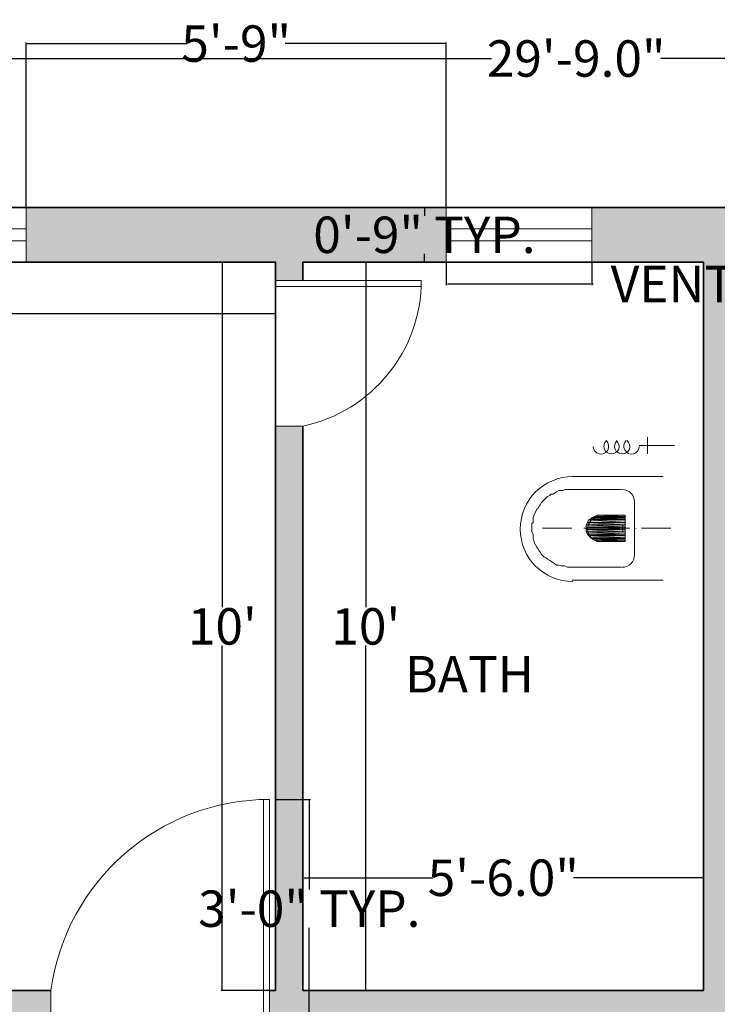
# Model space of a CAD drawing. Units: inches. Extents: x 302 to 1258, y 831 to 1373.
# Tile 4 of 13: x 455 to 569, y 1211 to 1373. Entities that reach past the tile are written whole.
import ezdxf

# ---------------------------------------------------------------- set-up
doc = ezdxf.new("R2010")
doc.units = ezdxf.units.IN
doc.header["$MEASUREMENT"] = 0
for name, color, linetype, lineweight in [('A-ANNO-DIMS', 2, 'Continuous', 18), ('A-AREA-IDEN', 7, 'Continuous', 18), ('A-DOOR', 3, 'Continuous', 18), ('A-FLOR-FIXT', 8, 'Continuous', 18), ('A-GLAZ', 4, 'Continuous', 18), ('A-WALL', 7, 'Continuous', 35), ('A-WALL-PATT', 251, 'Continuous', 13)]:
    doc.layers.add(name, color=color, linetype=linetype, lineweight=lineweight)
doc.styles.get("Standard").update_dxf_attribs({"font": 'arial.ttf'})
doc.dimstyles.get("Standard").update_dxf_attribs({"dimtxt": 6, "dimasz": 0.18, "dimexe": 0.18, "dimexo": 0.0625, "dimgap": 0.09, "dimtad": 0, "dimtih": 1, "dimtoh": 1, "dimdec": 1, "dimzin": 0, "dimdsep": 46, "dimlunit": 3, "dimtxsty": 'Standard', "dimcen": 0.09, "dimadec": 0, "dimazin": 0, "dimtfac": 1, "dimtdec": 1, "dimtofl": 0, "dimtmove": 0, "dimatfit": 3, "dimfxl": 1, "dimtolj": 1, "dimtzin": 0, "dimarcsym": 0})

# ---------------------------------------------------------------- blocks, each defined once
blk = doc.blocks.new('*D3')
at = {"layer": 'A-ANNO-DIMS', "color": 0, "lineweight": -2, "transparency": 16777216}
for p, q in [((376.67, 1333.26), (376.67, 1324.65)), ((496.67, 1333.26), (496.67, 1324.65)), ((376.85, 1324.83), (431.77, 1324.83)), ((496.49, 1324.83), (441.57, 1324.83))]:
    blk.add_line(p, q, dxfattribs=at)
at = {"layer": 'A-ANNO-DIMS', "color": 0, "transparency": 16777216}
for points in [[(376.85, 1324.86), (376.85, 1324.8), (376.67, 1324.83)], [(496.49, 1324.86), (496.49, 1324.8), (496.67, 1324.83)]]:
    blk.add_solid(points, dxfattribs=at)
at = {"layer": 'Defpoints', "color": 0, "transparency": 16777216}
for p in [(376.67, 1333.32), (496.67, 1333.32), (496.67, 1324.83)]:
    blk.add_point(p, dxfattribs=at)
at = {"layer": 'A-ANNO-DIMS', "color": 0, "transparency": 16777216, "insert": (436.67, 1324.83), "char_height": 6, "attachment_point": 5}
blk.add_mtext("\\A1;10'", dxfattribs=at)
blk = doc.blocks.new('*D4')
at = {"layer": 'A-ANNO-DIMS', "color": 0, "lineweight": -2, "transparency": 16777216}
for p, q in [((501.17, 1213.38), (501.17, 1232.1)), ((501.35, 1231.92), (522.61, 1231.92)), ((566.99, 1231.92), (545.73, 1231.92)), ((567.17, 1213.38), (567.17, 1232.1))]:
    blk.add_line(p, q, dxfattribs=at)
at = {"layer": 'A-ANNO-DIMS', "color": 0, "transparency": 16777216}
for points in [[(501.35, 1231.95), (501.35, 1231.89), (501.17, 1231.92)], [(566.99, 1231.95), (566.99, 1231.89), (567.17, 1231.92)]]:
    blk.add_solid(points, dxfattribs=at)
at = {"layer": 'Defpoints', "color": 0, "transparency": 16777216}
for p in [(567.17, 1231.92), (501.17, 1213.32), (567.17, 1213.32)]:
    blk.add_point(p, dxfattribs=at)
at = {"layer": 'A-ANNO-DIMS', "color": 0, "transparency": 16777216, "insert": (534.17, 1231.92), "char_height": 6, "attachment_point": 5}
blk.add_mtext('\\A1;5\'-6.0"', dxfattribs=at)
blk = doc.blocks.new('*D5')
at = {"layer": 'A-ANNO-DIMS', "color": 0, "lineweight": -2, "transparency": 16777216}
for p, q in [((496.61, 1333.32), (487.71, 1333.32)), ((487.89, 1333.14), (487.89, 1276.47)), ((487.89, 1213.5), (487.89, 1270.17)), ((496.61, 1213.32), (487.71, 1213.32))]:
    blk.add_line(p, q, dxfattribs=at)
at = {"layer": 'A-ANNO-DIMS', "color": 0, "transparency": 16777216}
for points in [[(487.86, 1333.14), (487.92, 1333.14), (487.89, 1333.32)], [(487.86, 1213.5), (487.92, 1213.5), (487.89, 1213.32)]]:
    blk.add_solid(points, dxfattribs=at)
at = {"layer": 'Defpoints', "color": 0, "transparency": 16777216}
for p in [(496.67, 1333.32), (487.89, 1213.32), (496.67, 1213.32)]:
    blk.add_point(p, dxfattribs=at)
at = {"layer": 'A-ANNO-DIMS', "color": 0, "transparency": 16777216, "insert": (487.89, 1273.32), "char_height": 6, "attachment_point": 5}
blk.add_mtext("\\A1;10'", dxfattribs=at)
blk = doc.blocks.new('*D6')
at = {"layer": 'A-ANNO-DIMS', "color": 0, "lineweight": -2, "transparency": 16777216}
for p, q in [((567.11, 1333.32), (511.34, 1333.32)), ((511.52, 1333.14), (511.52, 1276.47)), ((511.52, 1213.5), (511.52, 1270.17)), ((567.11, 1213.32), (511.34, 1213.32))]:
    blk.add_line(p, q, dxfattribs=at)
at = {"layer": 'A-ANNO-DIMS', "color": 0, "transparency": 16777216}
for points in [[(511.49, 1333.14), (511.55, 1333.14), (511.52, 1333.32)], [(511.49, 1213.5), (511.55, 1213.5), (511.52, 1213.32)]]:
    blk.add_solid(points, dxfattribs=at)
at = {"layer": 'Defpoints', "color": 0, "transparency": 16777216}
for p in [(567.17, 1333.32), (511.52, 1213.32), (567.17, 1213.32)]:
    blk.add_point(p, dxfattribs=at)
at = {"layer": 'A-ANNO-DIMS', "color": 0, "transparency": 16777216, "insert": (511.52, 1273.32), "char_height": 6, "attachment_point": 5}
blk.add_mtext("\\A1;10'", dxfattribs=at)
blk = doc.blocks.new('*D31')
at = {"layer": 'A-ANNO-DIMS', "color": 0, "lineweight": -2, "transparency": 16777216}
for p, q in [((367.67, 1342.38), (367.67, 1367.04)), ((367.85, 1366.86), (532.23, 1366.86)), ((724.49, 1366.86), (560.11, 1366.86)), ((724.67, 1342.38), (724.67, 1367.04))]:
    blk.add_line(p, q, dxfattribs=at)
at = {"layer": 'A-ANNO-DIMS', "color": 0, "transparency": 16777216}
for points in [[(367.85, 1366.89), (367.85, 1366.83), (367.67, 1366.86)], [(724.49, 1366.89), (724.49, 1366.83), (724.67, 1366.86)]]:
    blk.add_solid(points, dxfattribs=at)
at = {"layer": 'Defpoints', "color": 0, "transparency": 16777216}
for p in [(724.67, 1366.86), (367.67, 1342.32), (724.67, 1342.32)]:
    blk.add_point(p, dxfattribs=at)
at = {"layer": 'A-ANNO-DIMS', "color": 0, "transparency": 16777216, "insert": (546.17, 1366.86), "char_height": 6, "attachment_point": 5}
blk.add_mtext('\\A1;29\'-9.0"', dxfattribs=at)
blk = doc.blocks.new('WC-PLAN')
h = blk.add_hatch(color=256)
h.paths.add_polyline_path([(17.3, 10.16), (11.23, 10.16), (17.3, 9.71)])
h.paths.add_polyline_path([(11.23, 10.16), (17.3, 9.71), (11.08, 9.71)])
h = blk.add_hatch(color=256)
h.paths.add_polyline_path([(17.3, 10.32), (11.61, 10.32), (17.3, 10.16)])
h.paths.add_polyline_path([(11.61, 10.32), (17.3, 10.16), (11.23, 10.16)])
h = blk.add_hatch(color=256)
h.paths.add_polyline_path([(17.3, 10.54), (11.83, 10.54), (17.3, 10.32)])
h.paths.add_polyline_path([(11.83, 10.54), (17.3, 10.32), (11.61, 10.32)])
h = blk.add_hatch(color=256)
h.paths.add_polyline_path([(17.3, 10.7), (12.21, 10.7), (17.3, 10.54)])
h.paths.add_polyline_path([(12.21, 10.7), (17.3, 10.54), (11.83, 10.54)])
h = blk.add_hatch(color=256)
h.paths.add_polyline_path([(17.3, 10.92), (12.59, 10.92), (17.3, 10.7)])
h.paths.add_polyline_path([(12.59, 10.92), (17.3, 10.7), (12.21, 10.7)])
h = blk.add_hatch(color=256)
h.paths.add_polyline_path([(17.3, 9.71), (11.08, 9.71), (17.3, 9.33)])
h.paths.add_polyline_path([(11.08, 9.71), (17.3, 9.33), (10.85, 9.33)])
h = blk.add_hatch(color=256)
h.paths.add_polyline_path([(17.3, 9.33), (10.85, 9.33), (17.3, 8.95)])
h.paths.add_polyline_path([(10.85, 9.33), (17.3, 8.95), (10.85, 8.95)])
h = blk.add_hatch(color=256)
h.paths.add_polyline_path([(17.3, 8.95), (10.85, 8.95), (17.3, 8.57)])
h.paths.add_polyline_path([(10.85, 8.95), (17.3, 8.57), (10.85, 8.57)])
h = blk.add_hatch(color=256)
h.paths.add_polyline_path([(17.3, 8.57), (10.85, 8.57), (17.3, 8.19)])
h.paths.add_polyline_path([(10.85, 8.57), (17.3, 8.19), (10.85, 8.19)])
h = blk.add_hatch(color=256)
h.paths.add_polyline_path([(17.3, 8.19), (10.85, 8.19), (17.3, 7.81)])
h.paths.add_polyline_path([(10.85, 8.19), (17.3, 7.81), (11.08, 7.81)])
h = blk.add_hatch(color=256)
h.paths.add_polyline_path([(17.3, 7.81), (11.08, 7.81), (17.3, 7.59)])
h.paths.add_polyline_path([(11.08, 7.81), (17.3, 7.59), (11.23, 7.59)])
h = blk.add_hatch(color=256)
h.paths.add_polyline_path([(17.3, 7.59), (11.23, 7.59), (17.3, 7.21)])
h.paths.add_polyline_path([(11.23, 7.59), (17.3, 7.21), (11.61, 7.21)])
h = blk.add_hatch(color=256)
h.paths.add_polyline_path([(17.3, 7.21), (11.61, 7.21), (17.3, 7.05)])
h.paths.add_polyline_path([(11.61, 7.21), (17.3, 7.05), (11.83, 7.05)])
h = blk.add_hatch(color=256)
h.paths.add_polyline_path([(17.3, 7.05), (11.83, 7.05), (17.3, 6.83)])
h.paths.add_polyline_path([(11.83, 7.05), (17.3, 6.83), (12.21, 6.83)])
h = blk.add_hatch(color=256)
h.paths.add_polyline_path([(17.3, 6.83), (12.21, 6.83), (17.3, 6.6)])
h.paths.add_polyline_path([(12.21, 6.83), (17.3, 6.6), (12.59, 6.6)])
h.paths.add_polyline_path([(17.3, 6.6), (12.59, 6.6), (12.97, 6.6)])
for points in [[(20.94, 21.03), (20.94, 23.77), (20.94, 23.77)], [(25.41, 22.4), (19.57, 22.4), (19.57, 22.4)], [(23.52, 17.3), (8.5, 17.3), (8.5, 17.3)], [(9.48, 2.35), (8.72, 2.35), (8.12, 2.35), (7.74, 2.35), (7.36, 2.58), (6.98, 2.58), (6.75, 2.58), (6.37, 2.73), (5.99, 2.73), (5.61, 2.96), (5.39, 3.11), (5.01, 3.34), (4.85, 3.49), (4.48, 3.72), (4.25, 3.94), (3.87, 4.1), (3.64, 4.32), (3.49, 4.48), (3.26, 4.85), (3.11, 5.08), (2.88, 5.46), (2.73, 5.69), (2.5, 6.07), (2.28, 6.45), (2.28, 6.6), (2.12, 7.05), (2.12, 7.43), (2.12, 7.81), (1.9, 8.19), (1.9, 8.8), (1.9, 9.56), (2.12, 9.71), (2.12, 10.16), (2.12, 10.54), (2.28, 10.92), (2.28, 11.07), (2.5, 11.45), (2.73, 11.91), (2.88, 12.06), (3.11, 12.44), (3.26, 12.67), (3.49, 13.05), (3.64, 13.2), (3.87, 13.43), (4.25, 13.81), (4.48, 14.03), (4.85, 14.18), (5.01, 14.41), (5.39, 14.41), (5.61, 14.56), (5.99, 14.79), (6.37, 15.02), (6.75, 15.02), (6.98, 15.02), (7.36, 15.17), (7.74, 15.17), (8.12, 15.17), (8.72, 15.17), (9.48, 15.17)], [(16.69, 15.17), (9.48, 15.17), (9.48, 15.17)], [(18.81, 4.48), (18.81, 13.2), (18.81, 13.2)], [(17.3, 10.92), (12.97, 10.92), (12.97, 10.92)], [(17.3, 6.6), (17.3, 10.92), (17.3, 10.92)], [(8.5, 8.8), (3.64, 8.8), (3.64, 8.8)], [(18.05, 8.8), (10.47, 8.8), (10.47, 8.8)], [(16.84, 9.18), (16.92, 9.18), (16.92, 9.18)], [(16.84, 8.8), (16.84, 8.95), (16.84, 9.18)], [(16.84, 8.8), (16.92, 8.72), (16.92, 8.72)], [(16.84, 8.34), (16.84, 8.57), (16.84, 8.8)], [(16.84, 8.34), (16.92, 8.34), (16.92, 8.34)], [(19.04, 8.8), (19.04, 8.72), (19.04, 8.72)], [(24.81, 8.8), (19.95, 8.8), (19.95, 8.8)], [(17.3, 6.6), (12.97, 6.6), (12.97, 6.6)], [(16.69, 2.35), (9.48, 2.35), (9.48, 2.35)], [(23.52, 0.23), (8.5, 0.23), (8.5, 0.23)]]:
    blk.add_lwpolyline(points)
for points in [[(11.23, 10.16), (17.3, 9.71), (11.08, 9.71)], [(11.61, 10.32), (17.3, 10.16), (11.23, 10.16)], [(17.3, 10.16), (11.23, 10.16), (17.3, 9.71)], [(11.83, 10.54), (17.3, 10.32), (11.61, 10.32)], [(17.3, 10.32), (11.61, 10.32), (17.3, 10.16)], [(12.21, 10.7), (17.3, 10.54), (11.83, 10.54)], [(17.3, 10.54), (11.83, 10.54), (17.3, 10.32)], [(12.59, 10.92), (17.3, 10.7), (12.21, 10.7)], [(17.3, 10.7), (12.21, 10.7), (17.3, 10.54)], [(12.97, 10.92), (17.3, 10.92), (12.59, 10.92)], [(17.3, 10.92), (12.59, 10.92), (17.3, 10.7)], [(17.3, 10.92), (12.97, 10.92)], [(11.08, 9.71), (17.3, 9.33), (10.85, 9.33)], [(17.3, 9.33), (10.85, 9.33), (17.3, 8.95)], [(10.85, 9.33), (17.3, 8.95), (10.85, 8.95)], [(17.3, 8.95), (10.85, 8.95), (17.3, 8.57)], [(10.85, 8.95), (17.3, 8.57), (10.85, 8.57)], [(17.3, 8.57), (10.85, 8.57), (17.3, 8.19)], [(10.85, 8.57), (17.3, 8.19), (10.85, 8.19)], [(17.3, 8.19), (10.85, 8.19), (17.3, 7.81)], [(10.85, 8.19), (17.3, 7.81), (11.08, 7.81)], [(17.3, 9.71), (11.08, 9.71), (17.3, 9.33)], [(17.3, 7.81), (11.08, 7.81), (17.3, 7.59)], [(11.08, 7.81), (17.3, 7.59), (11.23, 7.59)], [(17.3, 7.59), (11.23, 7.59), (17.3, 7.21)], [(11.23, 7.59), (17.3, 7.21), (11.61, 7.21)], [(17.3, 7.21), (11.61, 7.21), (17.3, 7.05)], [(11.61, 7.21), (17.3, 7.05), (11.83, 7.05)], [(17.3, 7.05), (11.83, 7.05), (17.3, 6.83)], [(11.83, 7.05), (17.3, 6.83), (12.21, 6.83)], [(17.3, 6.83), (12.21, 6.83), (17.3, 6.6)], [(12.21, 6.83), (17.3, 6.6), (12.59, 6.6)], [(17.3, 6.6), (12.59, 6.6), (12.97, 6.6)], [(12.59, 6.6), (17.3, 6.6), (17.3, 6.6)]]:
    blk.add_lwpolyline(points, close=True)
for points, knots in [([(11.99, 22.25), (11.99, 21.72), (12.44, 21.19), (12.97, 21.03), (12.97, 21.03), (13.5, 20.88), (14.11, 21.19), (14.41, 21.64), (14.41, 21.64), (14.64, 22.17), (14.56, 22.78), (14.19, 23.16)], [0, 0, 0, 0, 0.083333, 0.083333, 0.083333, 0.083334, 0.166667, 0.166667, 0.166667, 0.166668, 1, 1, 1, 1]), ([(14.19, 23.23), (13.81, 22.86), (13.65, 22.32), (13.88, 21.79), (13.88, 21.79), (14.03, 21.34), (14.49, 21.03), (15.02, 21.03), (15.02, 21.03), (15.55, 21.03), (16.01, 21.34), (16.23, 21.79), (16.23, 21.79), (16.39, 22.32), (16.23, 22.86), (15.85, 23.23)], [0, 0, 0, 0, 0.0625, 0.0625, 0.0625, 0.062501, 0.125, 0.125, 0.125, 0.125001, 0.1875, 0.1875, 0.1875, 0.187501, 1, 1, 1, 1]), ([(15.93, 23.16), (15.55, 22.86), (15.4, 22.25), (15.63, 21.79), (15.63, 21.79), (15.78, 21.34), (16.31, 21.03), (16.76, 21.03), (16.76, 21.03), (17.3, 21.03), (17.75, 21.34), (17.98, 21.79), (17.98, 21.79), (18.13, 22.32), (17.98, 22.86), (17.6, 23.23)], [0, 0, 0, 0, 0.0625, 0.0625, 0.0625, 0.062501, 0.125, 0.125, 0.125, 0.125001, 0.1875, 0.1875, 0.1875, 0.187501, 1, 1, 1, 1]), ([(17.45, 23.23), (17.07, 22.86), (16.92, 22.17), (17.22, 21.72), (17.22, 21.72), (17.52, 21.19), (18.05, 20.88), (18.66, 21.03), (18.66, 21.03), (19.19, 21.19), (19.57, 21.72), (19.57, 22.25)], [0, 0, 0, 0, 0.083333, 0.083333, 0.083333, 0.083334, 0.166667, 0.166667, 0.166667, 0.166668, 1, 1, 1, 1]), ([(8.65, 17.3), (3.87, 17.3), (0, 13.43), (0, 8.65), (0, 8.65), (0, 3.87), (3.87, 0), (8.65, 0)], [0, 0, 0, 0, 0.125, 0.125, 0.125, 0.125001, 1, 1, 1, 1]), ([(13.12, 10.7), (11.99, 10.7), (11.08, 9.79), (11.08, 8.65), (11.08, 8.65), (11.08, 7.51), (11.99, 6.6), (13.12, 6.6)], [0, 0, 0, 0, 0.125, 0.125, 0.125, 0.125001, 1, 1, 1, 1])]:
    blk.add_open_spline(points, degree=3, knots=knots)
for points in [[(18.81, 13.12), (18.81, 14.26), (17.9, 15.17), (16.76, 15.17)], [(16.76, 2.35), (17.9, 2.35), (18.81, 3.26), (18.81, 4.4)]]:
    blk.add_open_spline(points, degree=3)
blk = doc.blocks.new('WINDOW-48IN')
for p, q in [((0, 0), (0, 9)), ((0, 9), (48, 9)), ((48, 9), (48, 0)), ((0, 5.5), (48, 5.5)), ((48, 3.5), (0, 3.5)), ((48, 0), (0, 0))]:
    blk.add_line(p, q)
blk = doc.blocks.new('VENT-WINDOW-24IN')
for p, q in [((0, 24), (9, 24)), ((0, 0), (0, 24)), ((3.5, 0), (3.5, 24)), ((5.5, 24), (5.5, 0)), ((9, 24), (9, 0)), ((9, 0), (0, 0))]:
    blk.add_line(p, q)
blk = doc.blocks.new('DOOR-36IN-BEDROOM')
for p, q in [((35, 36), (35, 0)), ((36, 0), (36, 36)), ((36, 36), (36, 0)), ((0, 0), (0, 4.5)), ((36, 0), (0, 0)), ((37, 0), (36, 0))]:
    blk.add_line(p, q)
blk.add_arc((36, -0.32), 36.32, 90, 172.3719)
blk = doc.blocks.new('DOOR-24IN-BATH')
for p, q in [((0, 27), (0, 24)), ((0, 24), (24, 24)), ((24, 24), (0, 24)), ((0, 24), (0, 0)), ((24, 23), (0, 23)), ((0, 0), (4.5, 0))]:
    blk.add_line(p, q)
blk.add_arc((-0.52, 24), 24.52, 281.8123, 0)
blk = doc.blocks.new('*D53')
at = {"layer": 'A-ANNO-DIMS', "color": 0, "lineweight": -2, "transparency": 16777216}
for p, q in [((524.78, 1333.26), (524.78, 1329.54)), ((548.78, 1333.26), (548.78, 1329.54)), ((524.96, 1329.72), (548.6, 1329.72)), ((548.78, 1329.72), (548.96, 1329.72))]:
    blk.add_line(p, q, dxfattribs=at)
at = {"layer": 'A-ANNO-DIMS', "color": 0, "transparency": 16777216}
for points in [[(524.96, 1329.75), (524.96, 1329.69), (524.78, 1329.72)], [(548.6, 1329.75), (548.6, 1329.69), (548.78, 1329.72)]]:
    blk.add_solid(points, dxfattribs=at)
at = {"layer": 'Defpoints', "color": 0, "transparency": 16777216}
for p in [(524.78, 1333.32), (548.78, 1333.32), (548.78, 1329.72)]:
    blk.add_point(p, dxfattribs=at)
at = {"layer": 'A-ANNO-DIMS', "color": 0, "transparency": 16777216, "insert": (599.38, 1329.72), "char_height": 6, "attachment_point": 5}
blk.add_mtext('\\A1;VENT WINDOW 2\'-0" TYP.', dxfattribs=at)
blk = doc.blocks.new('*D54')
at = {"layer": 'A-ANNO-DIMS', "color": 0, "lineweight": -2, "transparency": 16777216}
for p, q in [((524.71, 1342.32), (521, 1342.32)), ((521.18, 1342.14), (521.18, 1340.97)), ((524.71, 1333.32), (521, 1333.32)), ((521.18, 1333.5), (521.18, 1334.67))]:
    blk.add_line(p, q, dxfattribs=at)
at = {"layer": 'A-ANNO-DIMS', "color": 0, "transparency": 16777216}
for points in [[(521.15, 1342.14), (521.21, 1342.14), (521.18, 1342.32)], [(521.15, 1333.5), (521.21, 1333.5), (521.18, 1333.32)]]:
    blk.add_solid(points, dxfattribs=at)
at = {"layer": 'Defpoints', "color": 0, "transparency": 16777216}
for p in [(524.78, 1342.32), (521.18, 1333.32), (524.78, 1333.32)]:
    blk.add_point(p, dxfattribs=at)
at = {"layer": 'A-ANNO-DIMS', "color": 0, "transparency": 16777216, "insert": (521.18, 1337.82), "char_height": 6, "attachment_point": 5}
blk.add_mtext('\\A1;0\'-9" TYP.', dxfattribs=at)
blk = doc.blocks.new('*D55')
at = {"layer": 'A-ANNO-DIMS', "color": 0, "lineweight": -2, "transparency": 16777216}
for p, q in [((459.67, 1208.76), (459.67, 1203.09)), ((496.67, 1208.76), (496.67, 1203.09)), ((459.85, 1203.27), (496.49, 1203.27)), ((496.67, 1203.27), (496.85, 1203.27))]:
    blk.add_line(p, q, dxfattribs=at)
at = {"layer": 'A-ANNO-DIMS', "color": 0, "transparency": 16777216}
for points in [[(459.85, 1203.3), (459.85, 1203.24), (459.67, 1203.27)], [(496.49, 1203.3), (496.49, 1203.24), (496.67, 1203.27)]]:
    blk.add_solid(points, dxfattribs=at)
at = {"layer": 'Defpoints', "color": 0, "transparency": 16777216}
for p in [(459.67, 1208.82), (496.67, 1208.82), (496.67, 1203.27)]:
    blk.add_point(p, dxfattribs=at)
at = {"layer": 'A-ANNO-DIMS', "color": 0, "transparency": 16777216, "insert": (551.65, 1203.27), "char_height": 6, "attachment_point": 5}
blk.add_mtext('\\A1;BEDROOM DOOR 3\'-1" TYP.', dxfattribs=at)
blk = doc.blocks.new('*D56')
at = {"layer": 'A-ANNO-DIMS', "color": 0, "lineweight": -2, "transparency": 16777216}
for p, q in [((496.73, 1244.82), (502.4, 1244.82)), ((502.22, 1244.64), (502.22, 1229.97)), ((502.22, 1209), (502.22, 1223.66)), ((496.73, 1208.82), (502.4, 1208.82))]:
    blk.add_line(p, q, dxfattribs=at)
at = {"layer": 'A-ANNO-DIMS', "color": 0, "transparency": 16777216}
for points in [[(502.19, 1244.64), (502.25, 1244.64), (502.22, 1244.82)], [(502.19, 1209), (502.25, 1209), (502.22, 1208.82)]]:
    blk.add_solid(points, dxfattribs=at)
at = {"layer": 'Defpoints', "color": 0, "transparency": 16777216}
for p in [(496.67, 1244.82), (502.22, 1244.82), (496.67, 1208.82)]:
    blk.add_point(p, dxfattribs=at)
at = {"layer": 'A-ANNO-DIMS', "color": 0, "transparency": 16777216, "insert": (502.22, 1226.82), "char_height": 6, "attachment_point": 5}
blk.add_mtext('\\A1;3\'-0" TYP.', dxfattribs=at)
blk = doc.blocks.new('*D70')
at = {"layer": 'A-ANNO-DIMS', "color": 0, "lineweight": -2, "transparency": 16777216}
for p, q in [((455.57, 1342.38), (455.57, 1369.5)), ((455.75, 1369.32), (482.11, 1369.32)), ((524.6, 1369.32), (498.24, 1369.32)), ((524.78, 1342.38), (524.78, 1369.5))]:
    blk.add_line(p, q, dxfattribs=at)
at = {"layer": 'A-ANNO-DIMS', "color": 0, "transparency": 16777216}
for points in [[(455.75, 1369.35), (455.75, 1369.29), (455.57, 1369.32)], [(524.6, 1369.35), (524.6, 1369.29), (524.78, 1369.32)]]:
    blk.add_solid(points, dxfattribs=at)
at = {"layer": 'Defpoints', "color": 0, "transparency": 16777216}
for p in [(524.78, 1369.32), (455.57, 1342.32), (524.78, 1342.32)]:
    blk.add_point(p, dxfattribs=at)
at = {"layer": 'A-ANNO-DIMS', "color": 0, "transparency": 16777216, "insert": (490.18, 1369.32), "char_height": 6, "attachment_point": 5}
blk.add_mtext('\\A1;5\'-9"', dxfattribs=at)

msp = doc.modelspace()

# ---------------------------------------------------------------- hatches: boundary and pattern name
at = {"layer": 'A-WALL-PATT'}
h = msp.add_hatch(color=256, dxfattribs=at)
h.dxf.hatch_style = 1
h.paths.add_polyline_path([(524.78, 1342.32), (455.57, 1342.32), (455.57, 1333.32), (496.67, 1333.32), (496.67, 1330.32), (501.17, 1330.32), (501.17, 1333.32), (524.78, 1333.32)])
h.paths.add_polyline_path([(724.67, 1342.32), (548.78, 1342.32), (548.78, 1333.32), (567.17, 1333.32), (567.17, 1213.32), (501.17, 1213.32), (501.17, 1306.32), (496.67, 1306.32), (496.67, 1213.32), (495.67, 1213.32), (495.67, 1208.82), (496.67, 1208.82), (572.67, 1208.82), (572.67, 1213.32), (571.67, 1213.32), (571.67, 1333.32), (715.67, 1333.32), (715.67, 1302.71), (724.67, 1302.71)])
h.paths.add_polyline_path([(376.67, 1333.32), (407.57, 1333.32), (407.57, 1342.32), (367.67, 1342.32), (367.67, 1300.76), (376.67, 1300.76)])
h.paths.add_polyline_path([(459.67, 1213.32), (376.67, 1213.32), (376.67, 1252.76), (367.67, 1252.76), (367.67, 1164.55), (376.67, 1164.55), (376.67, 1208.82), (454.67, 1208.82), (454.67, 1082.82), (459.17, 1082.82), (459.17, 1208.82), (459.67, 1208.82)])
h.paths.add_polyline_path([(376.67, 1116.55), (367.67, 1116.55), (367.67, 1024.44), (376.67, 1024.44)])
h.paths.add_polyline_path([(724.67, 1254.71), (715.67, 1254.71), (715.67, 1213.32), (608.67, 1213.32), (608.67, 1208.82), (615.17, 1208.82), (615.17, 1205.82), (619.67, 1205.82), (619.67, 1208.82), (715.67, 1208.82), (715.67, 1191.3), (724.67, 1191.3)])
h.paths.add_polyline_path([(724.67, 1167.3), (715.67, 1167.3), (715.67, 1136.82), (619.67, 1136.82), (619.67, 1181.82), (615.17, 1181.82), (615.17, 1136.82), (591.17, 1136.82), (591.17, 1129.32), (595.67, 1129.32), (595.67, 1132.32), (715.67, 1132.32), (715.67, 1097.42), (724.67, 1097.42)])
h.paths.add_polyline_path([(724.67, 1049.42), (715.67, 1049.42), (715.67, 1012.32), (595.67, 1012.32), (595.67, 1093.32), (591.17, 1093.32), (591.17, 1007.82), (715.67, 1007.82), (715.67, 875.82), (709.67, 875.82), (709.67, 866.82), (715.67, 866.82), (724.67, 866.82)])
h.paths.add_polyline_path([(673.67, 875.82), (623.88, 875.82), (623.88, 866.82), (673.67, 866.82)], flags=17)
h.paths.add_polyline_path([(575.88, 875.82), (477.17, 875.82), (477.17, 971.82), (472.67, 971.82), (472.67, 875.82), (376.67, 875.82), (376.67, 896.2), (367.67, 896.2), (367.67, 866.82), (575.88, 866.82)])
h.paths.add_polyline_path([(376.67, 976.44), (367.67, 976.44), (367.67, 944.2), (376.67, 944.2)])

# ---------------------------------------------------------------- linework, layer by layer
at = {"layer": 'A-WALL'}
for p, q in [((367.67, 1342.32), (724.67, 1342.32)), ((376.67, 1333.32), (496.67, 1333.32)), ((496.67, 1333.32), (496.67, 1213.32)), ((501.17, 1333.32), (501.17, 1330.32)), ((501.17, 1333.32), (567.17, 1333.32)), ((567.17, 1333.32), (567.17, 1213.32)), ((501.17, 1306.32), (501.17, 1213.32)), ((376.67, 1213.32), (459.67, 1213.32)), ((495.67, 1213.32), (496.67, 1213.32)), ((501.17, 1213.32), (567.17, 1213.32))]:
    msp.add_line(p, q, dxfattribs=at)

# ---------------------------------------------------------------- block references
at = {"layer": 'A-DOOR'}
for name, p in [('DOOR-24IN-BATH', (496.67, 1306.32)), ('DOOR-36IN-BEDROOM', (459.67, 1208.82))]:
    msp.add_blockref(name, p, dxfattribs=at)
at = {"layer": 'A-FLOR-FIXT'}
msp.add_blockref('WC-PLAN', (536.97, 1280.7), dxfattribs=at)
at = {"layer": 'A-GLAZ'}
msp.add_blockref('WINDOW-48IN', (407.57, 1333.32), dxfattribs=at)
at = {"layer": 'A-GLAZ', "rotation": 269.9999999999994}
msp.add_blockref('VENT-WINDOW-24IN', (524.78, 1342.32), dxfattribs=at)

# ---------------------------------------------------------------- texts
at = {"layer": 'A-AREA-IDEN', "insert": (518, 1268.44), "char_height": 6, "attachment_point": 1}
msp.add_mtext_dynamic_manual_height_columns('BATH', width=33.1895, gutter_width=30, heights=[0], dxfattribs=at)

# ---------------------------------------------------------------- dimensions: what is measured, and where the dimension line sits
at = {"layer": 'A-ANNO-DIMS'}
for base, p1, p2, override, picture, middle in [((524.78, 1369.32), (455.57, 1342.32), (524.78, 1342.32), {"dimdec": 1, "dimlfac": 1, "dimrnd": 0, "dimzin": 1, "dimdsep": 46, "dimlunit": 4, "dimfrac": 2}, '*D70', (490.18, 1369.32)), ((724.67, 1366.86), (367.67, 1342.32), (724.67, 1342.32), {"dimclrd": 0, "dimclre": 0, "dimclrt": 0}, '*D31', (546.17, 1366.86)), ((496.67, 1324.83), (376.67, 1333.32), (496.67, 1333.32), {"dimclrd": 0, "dimclre": 0, "dimclrt": 0}, '*D3', (436.67, 1324.83)), ((567.17, 1231.92), (501.17, 1213.32), (567.17, 1213.32), {"dimclrd": 0, "dimclre": 0, "dimclrt": 0}, '*D4', (534.17, 1231.92))]:
    dim = msp.add_linear_dim(base=base, p1=p1, p2=p2, dimstyle='Standard', override=override, dxfattribs=at)
    dim.commit()
    dim.dimension.update_dxf_attribs({"geometry": picture, "text_midpoint": middle})
for base, p1, p2, text, picture, middle in [((548.78, 1329.72), (524.78, 1333.32), (548.78, 1333.32), 'VENT WINDOW <> TYP.', '*D53', (599.38, 1329.72)), ((496.67, 1203.27), (459.67, 1208.82), (496.67, 1208.82), 'BEDROOM DOOR <> TYP.', '*D55', (551.65, 1203.27))]:
    dim = msp.add_linear_dim(base=base, p1=p1, p2=p2, text=text, dimstyle='Standard', override={"dimdec": 1, "dimlfac": 1, "dimrnd": 0, "dimzin": 1, "dimdsep": 46, "dimlunit": 4, "dimfrac": 2}, dxfattribs=at)
    dim.commit()
    dim.dimension.update_dxf_attribs({"geometry": picture, "text_midpoint": middle})
for base, p1, p2, angle, picture, middle in [((521.18, 1333.32), (524.78, 1342.32), (524.78, 1333.32), 270, '*D54', (521.18, 1337.82)), ((502.22, 1244.82), (496.67, 1208.82), (496.67, 1244.82), 90, '*D56', (502.22, 1226.82))]:
    dim = msp.add_linear_dim(base=base, p1=p1, p2=p2, angle=angle, text='<> TYP.', dimstyle='Standard', override={"dimdec": 1, "dimlfac": 1, "dimrnd": 0, "dimzin": 1, "dimdsep": 46, "dimlunit": 4, "dimfrac": 2}, dxfattribs=at)
    dim.commit()
    dim.dimension.update_dxf_attribs({"geometry": picture, "text_midpoint": middle})
for base, p1, p2, picture, middle in [((487.89, 1213.32), (496.67, 1333.32), (496.67, 1213.32), '*D5', (487.89, 1273.32)), ((511.52, 1213.32), (567.17, 1333.32), (567.17, 1213.32), '*D6', (511.52, 1273.32))]:
    dim = msp.add_linear_dim(base=base, p1=p1, p2=p2, angle=90, dimstyle='Standard', override={"dimclrd": 0, "dimclre": 0, "dimclrt": 0}, dxfattribs=at)
    dim.commit()
    dim.dimension.update_dxf_attribs({"geometry": picture, "text_midpoint": middle})

doc.saveas('drawing.dxf')
